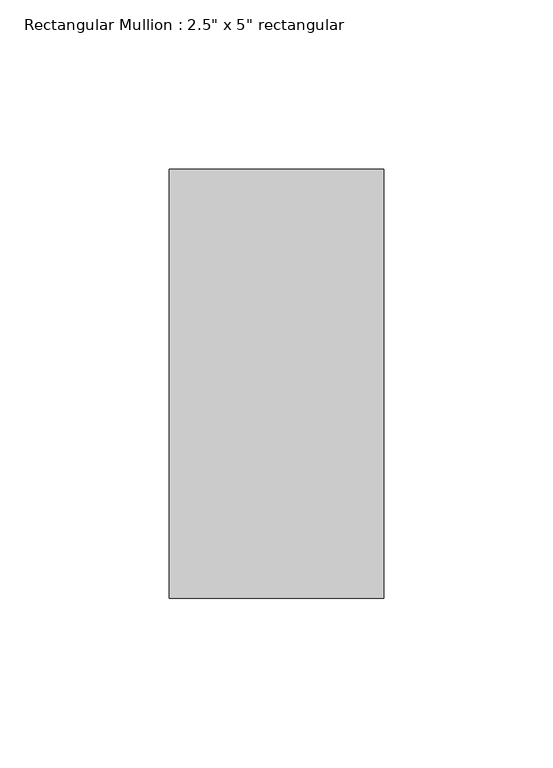
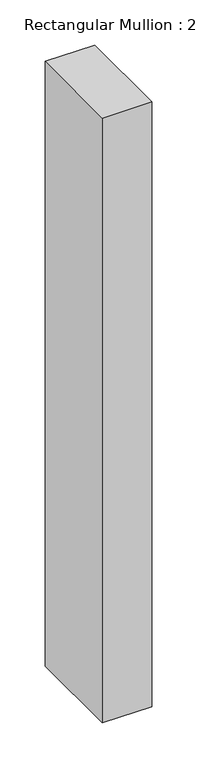
"""IFC4 building model written with IfcOpenShell, lengths in millimetres: member geometry."""

from ifc_helpers import new_model, si_unit, frame, origin, place, context, project, spatial, polyline, outline, extrude, source, transform, mapped, element, save


def member_ad567e07(model_context):
    return source(origin(), model_context, "Body", "SweptSolid", [
        extrude(outline(polyline([(31.75, 63.5), (31.75, -63.5), (-31.75, -63.5), (-31.75, 63.5), (31.75, 63.5)])), frame((0.0, 0.0, -819.15), z_axis=(0.0, 0.0, 1.0), x_axis=(1.0, 0.0, 0.0)), (0.0, 0.0, 1.0), 819.15),
    ])


if __name__ == "__main__":
    model = new_model("IFC4")
    model_context = context("Model", 3, world=origin())
    ifc_project = project(units=[si_unit("LENGTHUNIT", "METRE", prefix="MILLI")], contexts=[model_context])
    site = spatial("IfcSite", under=ifc_project)
    building = spatial("IfcBuilding", under=site)
    placement = place(None, origin())
    member_shape = member_ad567e07(model_context)
    element("IfcMember", 1, ObjectType="Rectangular Mullion : 2.5\" x 5\" rectangular", at=placement, inside=building, context=model_context, shape_type="MappedRepresentation", body=[
        mapped(member_shape, transform((0.0, 0.0, 0.0), x_axis=(1.0, 0.0, 0.0), y_axis=(0.0, 1.0, 0.0), z_axis=(0.0, 0.0, 1.0))),
    ])
    save(model, "model.ifc")

# Revit data of these elements
# Type "Rectangular Mullion : 2.5\" x 5\" rectangular"
#   built-in parameter 1007304 = 0.416667 (stored number, unit not read)
#   built-in parameter 1007301 = 0.104167 (stored number, unit not read)
#   built-in parameter 1007300 = 0.104167 (stored number, unit not read)
# Element 1 (IfcMember, "Rectangular Mullion : 2.5\" x 5\" rectangular")
#   Materials on its faces: "Iron, Ductile"
# Materials
#   "Iron, Ductile": class "Metal", colour RGB 0 0 0, transparency 0, Description = "Ductile cast iron", Cost = 0
